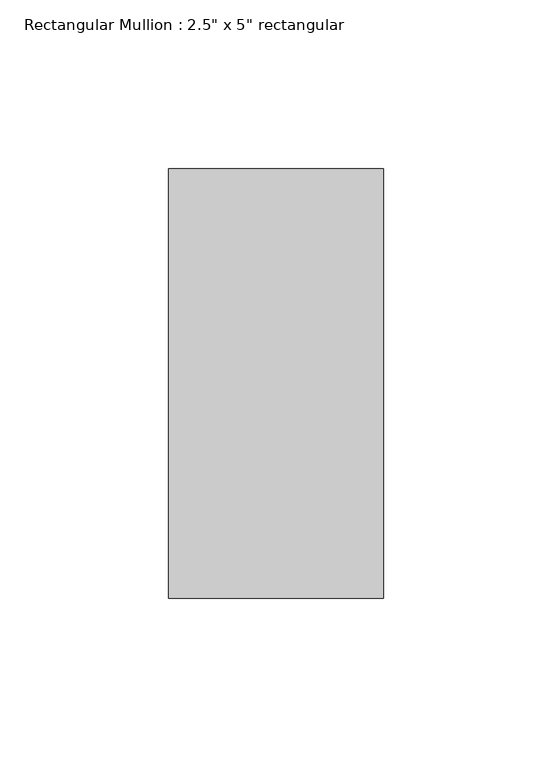
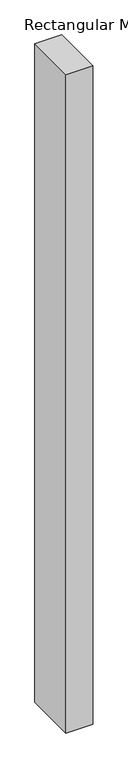
"""IFC4 building model written with IfcOpenShell, lengths in millimetres: member geometry."""

from ifc_helpers import new_model, si_unit, frame, origin, place, context, project, spatial, polyline, outline, extrude, source, transform, mapped, element, save


def member_66b74061(model_context):
    return source(origin(), model_context, "Body", "SweptSolid", [
        extrude(outline(polyline([(31.75, 63.5), (31.75, -63.5), (-31.75, -63.5), (-31.75, 63.5), (31.75, 63.5)])), frame((0.0, 0.0, -1645.1858302), z_axis=(0.0, 0.0, 1.0), x_axis=(1.0, 0.0, 0.0)), (0.0, 0.0, 1.0), 1645.1858302),
    ])


if __name__ == "__main__":
    model = new_model("IFC4")
    model_context = context("Model", 3, world=origin())
    ifc_project = project(units=[si_unit("LENGTHUNIT", "METRE", prefix="MILLI")], contexts=[model_context])
    site = spatial("IfcSite", under=ifc_project)
    building = spatial("IfcBuilding", under=site)
    placement = place(None, origin())
    member_shape = member_66b74061(model_context)
    element("IfcMember", 1, ObjectType="Rectangular Mullion : 2.5\" x 5\" rectangular", at=placement, inside=building, context=model_context, shape_type="MappedRepresentation", body=[
        mapped(member_shape, transform((0.0, 0.0, 0.0), x_axis=(1.0, 0.0, 0.0), y_axis=(0.0, 1.0, 0.0), z_axis=(0.0, 0.0, 1.0))),
    ])
    save(model, "model.ifc")

# Revit data of these elements
# Type "Rectangular Mullion : 2.5\" x 5\" rectangular"
#   built-in parameter 1007304 = 0.416667 (stored number, unit not read)
#   built-in parameter 1007301 = 0.104167 (stored number, unit not read)
#   built-in parameter 1007300 = 0.104167 (stored number, unit not read)
# Element 1 (IfcMember, "Rectangular Mullion : 2.5\" x 5\" rectangular")
#   Materials on its faces: "Aluminum"
# Materials
#   "Aluminum": class "Metal", colour RGB 247 247 247, transparency 0, Description = "Aluminum 6061", Cost = 0
